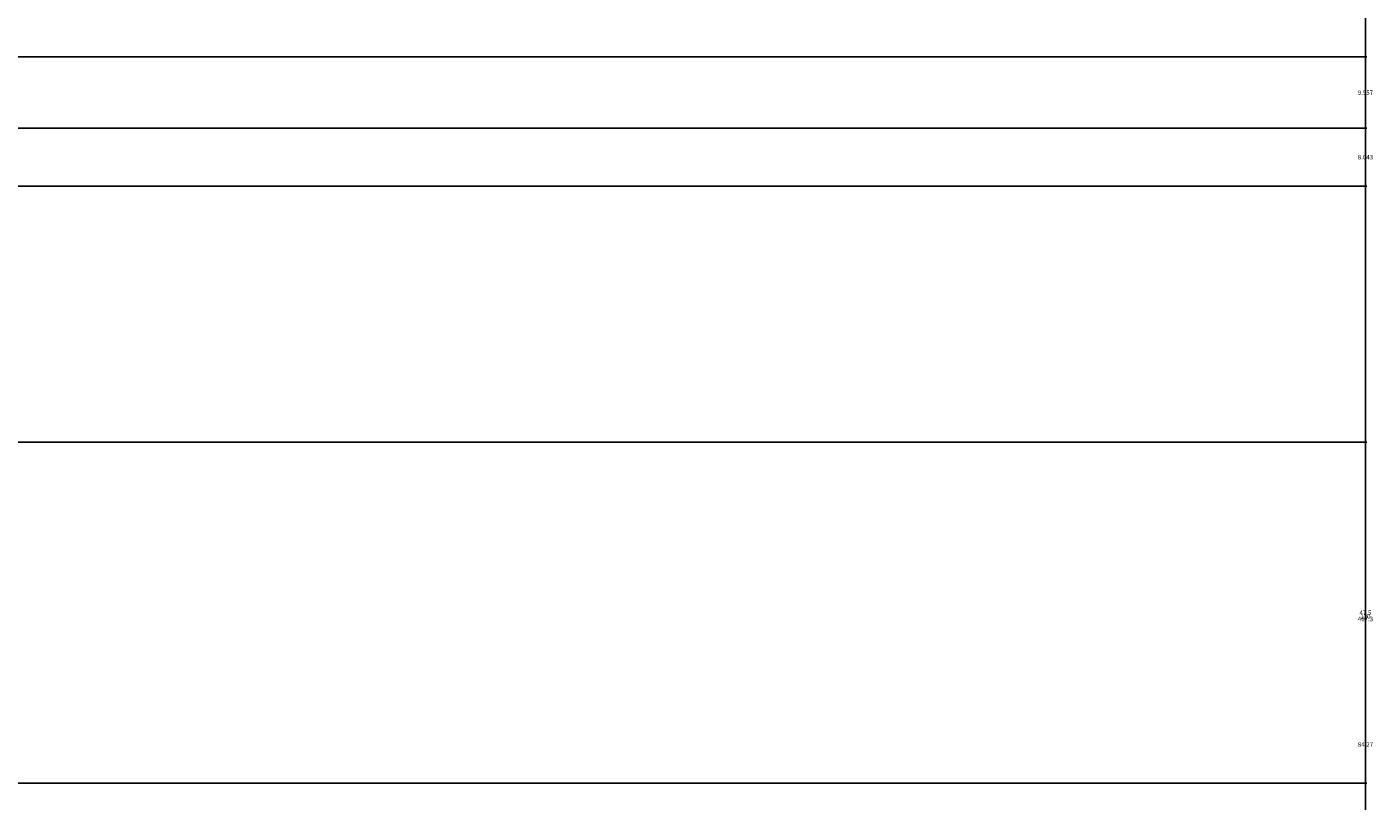
# Model space of a CAD drawing. Units: inches. Extents: x -13 to 809, y 112 to 656.
# Tile 51 of 55: x 621 to 809, y 359 to 467. Entities that reach past the tile are written whole.
import ezdxf

# ---------------------------------------------------------------- set-up
doc = ezdxf.new("R2010")
doc.units = ezdxf.units.IN
doc.header["$MEASUREMENT"] = 0
doc.layers.add('A-ANNO-DIMS', color=2, linetype='Continuous', lineweight=18)
doc.styles.get("Standard").update_dxf_attribs({"font": 'arial.ttf'})
doc.dimstyles.get("Standard").update_dxf_attribs({"dimtxt": 0.625, "dimasz": 0.18, "dimexe": 0.18, "dimexo": 0.0625, "dimgap": 0.09, "dimtad": 0, "dimtih": 1, "dimtoh": 1, "dimdec": 4, "dimzin": 0, "dimdsep": 46, "dimlunit": 4, "dimtxsty": 'Standard', "dimcen": 0.09, "dimadec": 0, "dimazin": 0, "dimtfac": 1, "dimtdec": 4, "dimtofl": 0, "dimtmove": 0, "dimatfit": 3, "dimfxl": 1, "dimtolj": 1, "dimtzin": 0, "dimarcsym": 0})

# ---------------------------------------------------------------- blocks, each defined once
blk = doc.blocks.new('*D31')
at = {"layer": 'A-ANNO-DIMS', "color": 0, "lineweight": -2, "transparency": 16777216}
for p, q in [((621.07, 617.78), (807.77, 617.78)), ((807.59, 617.6), (807.59, 384.56)), ((807.59, 150.7), (807.59, 383.74)), ((621.07, 150.52), (807.77, 150.52))]:
    blk.add_line(p, q, dxfattribs=at)
at = {"layer": 'A-ANNO-DIMS', "color": 0, "transparency": 16777216}
for points in [[(807.56, 617.6), (807.62, 617.6), (807.59, 617.78)], [(807.56, 150.7), (807.62, 150.7), (807.59, 150.52)]]:
    blk.add_solid(points, dxfattribs=at)
at = {"layer": 'Defpoints', "color": 0, "transparency": 16777216}
for p in [(621.01, 617.78), (807.59, 617.78), (621.01, 150.52)]:
    blk.add_point(p, dxfattribs=at)
at = {"layer": 'A-ANNO-DIMS', "color": 0, "transparency": 16777216, "insert": (807.59, 384.15), "char_height": 0.625, "attachment_point": 5}
blk.add_mtext('\\A1;467.3', dxfattribs=at)
blk = doc.blocks.new('*D46')
at = {"layer": 'A-ANNO-DIMS', "color": 0, "lineweight": -2, "transparency": 16777216}
for p, q in [((160.98, 408.79), (807.77, 408.79)), ((807.59, 408.61), (807.59, 367.07)), ((807.59, 324.7), (807.59, 366.25)), ((160.98, 324.52), (807.77, 324.52))]:
    blk.add_line(p, q, dxfattribs=at)
at = {"layer": 'A-ANNO-DIMS', "color": 0, "transparency": 16777216}
for points in [[(807.56, 408.61), (807.62, 408.61), (807.59, 408.79)], [(807.56, 324.7), (807.62, 324.7), (807.59, 324.52)]]:
    blk.add_solid(points, dxfattribs=at)
at = {"layer": 'Defpoints', "color": 0, "transparency": 16777216}
for p in [(160.92, 408.79), (807.59, 408.79), (160.92, 324.52)]:
    blk.add_point(p, dxfattribs=at)
at = {"layer": 'A-ANNO-DIMS', "color": 0, "transparency": 16777216, "insert": (807.59, 366.66), "char_height": 0.625, "attachment_point": 5}
blk.add_mtext('\\A1;84.27', dxfattribs=at)
blk = doc.blocks.new('*D47')
at = {"layer": 'A-ANNO-DIMS', "color": 0, "lineweight": -2, "transparency": 16777216}
for p, q in [((275.78, 408.79), (807.77, 408.79)), ((807.59, 408.61), (807.59, 385.45)), ((807.59, 361.47), (807.59, 384.63)), ((275.78, 361.29), (807.77, 361.29))]:
    blk.add_line(p, q, dxfattribs=at)
at = {"layer": 'A-ANNO-DIMS', "color": 0, "transparency": 16777216}
for points in [[(807.56, 408.61), (807.62, 408.61), (807.59, 408.79)], [(807.56, 361.47), (807.62, 361.47), (807.59, 361.29)]]:
    blk.add_solid(points, dxfattribs=at)
at = {"layer": 'Defpoints', "color": 0, "transparency": 16777216}
for p in [(275.71, 408.79), (807.59, 408.79), (275.71, 361.29)]:
    blk.add_point(p, dxfattribs=at)
at = {"layer": 'A-ANNO-DIMS', "color": 0, "transparency": 16777216, "insert": (807.59, 385.04), "char_height": 0.625, "attachment_point": 5}
blk.add_mtext('\\A1;47.5', dxfattribs=at)
blk = doc.blocks.new('*D48')
at = {"layer": 'A-ANNO-DIMS', "color": 0, "lineweight": -2, "transparency": 16777216}
for p, q in [((319.57, 444.52), (807.77, 444.52)), ((807.59, 444.34), (807.59, 384.93)), ((807.59, 324.7), (807.59, 384.11)), ((319.57, 324.52), (807.77, 324.52))]:
    blk.add_line(p, q, dxfattribs=at)
at = {"layer": 'A-ANNO-DIMS', "color": 0, "transparency": 16777216}
for points in [[(807.56, 444.34), (807.62, 444.34), (807.59, 444.52)], [(807.56, 324.7), (807.62, 324.7), (807.59, 324.52)]]:
    blk.add_solid(points, dxfattribs=at)
at = {"layer": 'Defpoints', "color": 0, "transparency": 16777216}
for p in [(319.51, 444.52), (807.59, 444.52), (319.51, 324.52)]:
    blk.add_point(p, dxfattribs=at)
at = {"layer": 'A-ANNO-DIMS', "color": 0, "transparency": 16777216, "insert": (807.59, 384.52), "char_height": 0.625, "attachment_point": 5}
blk.add_mtext('\\A1;120', dxfattribs=at)
blk = doc.blocks.new('*D104')
at = {"layer": 'A-ANNO-DIMS', "color": 0, "lineweight": -2, "transparency": 16777216}
for p, q in [((337.57, 462.52), (807.77, 462.52)), ((807.59, 462.34), (807.59, 457.95)), ((807.59, 452.74), (807.59, 457.13)), ((319.76, 452.56), (807.77, 452.56))]:
    blk.add_line(p, q, dxfattribs=at)
at = {"layer": 'A-ANNO-DIMS', "color": 0, "transparency": 16777216}
for points in [[(807.56, 462.34), (807.62, 462.34), (807.59, 462.52)], [(807.56, 452.74), (807.62, 452.74), (807.59, 452.56)]]:
    blk.add_solid(points, dxfattribs=at)
at = {"layer": 'Defpoints', "color": 0, "transparency": 16777216}
for p in [(337.51, 462.52), (319.7, 452.56), (807.59, 452.56)]:
    blk.add_point(p, dxfattribs=at)
at = {"layer": 'A-ANNO-DIMS', "color": 0, "transparency": 16777216, "insert": (807.59, 457.54), "char_height": 0.625, "attachment_point": 5}
blk.add_mtext('\\A1;9.957', dxfattribs=at)
blk = doc.blocks.new('*D105')
at = {"layer": 'A-ANNO-DIMS', "color": 0, "lineweight": -2, "transparency": 16777216}
for p, q in [((319.76, 452.56), (807.77, 452.56)), ((807.59, 452.38), (807.59, 448.95)), ((807.59, 444.7), (807.59, 448.13)), ((319.57, 444.52), (807.77, 444.52))]:
    blk.add_line(p, q, dxfattribs=at)
at = {"layer": 'A-ANNO-DIMS', "color": 0, "transparency": 16777216}
for points in [[(807.56, 452.38), (807.62, 452.38), (807.59, 452.56)], [(807.56, 444.7), (807.62, 444.7), (807.59, 444.52)]]:
    blk.add_solid(points, dxfattribs=at)
at = {"layer": 'Defpoints', "color": 0, "transparency": 16777216}
for p in [(319.7, 452.56), (319.51, 444.52), (807.59, 444.52)]:
    blk.add_point(p, dxfattribs=at)
at = {"layer": 'A-ANNO-DIMS', "color": 0, "transparency": 16777216, "insert": (807.59, 448.54), "char_height": 0.625, "attachment_point": 5}
blk.add_mtext('\\A1;8.043', dxfattribs=at)

msp = doc.modelspace()

# ---------------------------------------------------------------- dimensions: what is measured, and where the dimension line sits
at = {"layer": 'A-ANNO-DIMS'}
for base, p1, p2, override, picture, middle in [((807.5888, 617.7828), (621.008, 150.5199), (621.008, 617.7828), {"dimdec": 1, "dimlfac": 1, "dimrnd": 0, "dimzin": 0, "dimdsep": 46, "dimlunit": 2}, '*D31', (807.5888, 384.1514)), ((807.5888, 452.5629), (337.5074, 462.5199), (319.7004, 452.5629), {"dimdec": 3, "dimlfac": 1, "dimrnd": 0, "dimzin": 0, "dimdsep": 46, "dimlunit": 2}, '*D104', (807.5888, 457.5414)), ((807.5888, 444.5199), (319.7004, 452.5629), (319.5074, 444.5199), {"dimdec": 3, "dimlfac": 1, "dimrnd": 0, "dimzin": 0, "dimdsep": 46, "dimlunit": 2}, '*D105', (807.5888, 448.5414)), ((807.5888, 444.5199), (319.5074, 324.5199), (319.5074, 444.5199), {"dimdec": 0, "dimlfac": 1, "dimrnd": 0, "dimzin": 0, "dimdsep": 46, "dimlunit": 2}, '*D48', (807.5888, 384.5199)), ((807.5888, 408.7939), (160.9184, 324.5199), (160.9184, 408.7939), {"dimdec": 2, "dimlfac": 1, "dimrnd": 0, "dimzin": 0, "dimdsep": 46, "dimlunit": 2}, '*D46', (807.5888, 366.6569)), ((807.5888, 408.7939), (275.7145, 361.2915), (275.7145, 408.7939), {"dimdec": 1, "dimlfac": 1, "dimrnd": 0, "dimzin": 0, "dimdsep": 46, "dimlunit": 2}, '*D47', (807.5888, 385.0427))]:
    dim = msp.add_linear_dim(base=base, p1=p1, p2=p2, angle=90, dimstyle='Standard', override=override, dxfattribs=at)
    dim.commit()
    dim.dimension.update_dxf_attribs({"geometry": picture, "text_midpoint": middle})

doc.saveas('drawing.dxf')
